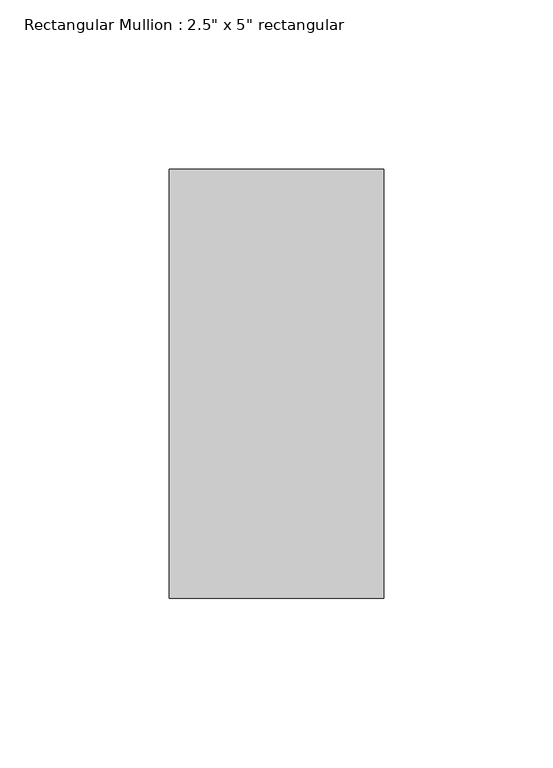
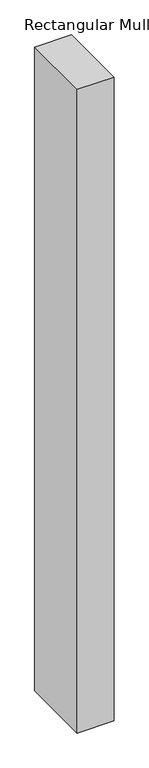
"""IFC4 building model written with IfcOpenShell, lengths in millimetres: member geometry."""

from ifc_helpers import new_model, si_unit, frame, origin, place, context, project, spatial, polyline, outline, extrude, source, transform, mapped, element, save


def member_5d96a33e(model_context):
    return source(origin(), model_context, "Body", "SweptSolid", [
        extrude(outline(polyline([(0.0, 63.5), (0.0, -63.5), (-63.5, -63.5), (-63.5, 63.5), (0.0, 63.5)])), frame((0.0, 0.0, -1174.7500001), z_axis=(0.0, 0.0, 1.0), x_axis=(1.0, 0.0, 0.0)), (0.0, 0.0, 1.0), 1174.7500001),
    ])


if __name__ == "__main__":
    model = new_model("IFC4")
    model_context = context("Model", 3, world=origin())
    ifc_project = project(units=[si_unit("LENGTHUNIT", "METRE", prefix="MILLI")], contexts=[model_context])
    site = spatial("IfcSite", under=ifc_project)
    building = spatial("IfcBuilding", under=site)
    placement = place(None, origin())
    member_shape = member_5d96a33e(model_context)
    element("IfcMember", 1, ObjectType="Rectangular Mullion : 2.5\" x 5\" rectangular", at=placement, inside=building, context=model_context, shape_type="MappedRepresentation", body=[
        mapped(member_shape, transform((0.0, 0.0, 0.0), x_axis=(1.0, 0.0, 0.0), y_axis=(0.0, 1.0, 0.0), z_axis=(0.0, 0.0, 1.0))),
    ])
    save(model, "model.ifc")

# Revit data of these elements
# Type "Rectangular Mullion : 2.5\" x 5\" rectangular"
#   built-in parameter 1007304 = 0.416667 (stored number, unit not read)
#   built-in parameter 1007301 = 0.104167 (stored number, unit not read)
#   built-in parameter 1007300 = 0.104167 (stored number, unit not read)
# Element 1 (IfcMember, "Rectangular Mullion : 2.5\" x 5\" rectangular")
#   Materials on its faces: "Aluminum"
# Materials
#   "Aluminum": class "Metal", colour RGB 247 247 247, transparency 0, Description = "Aluminum 6061", Cost = 0
